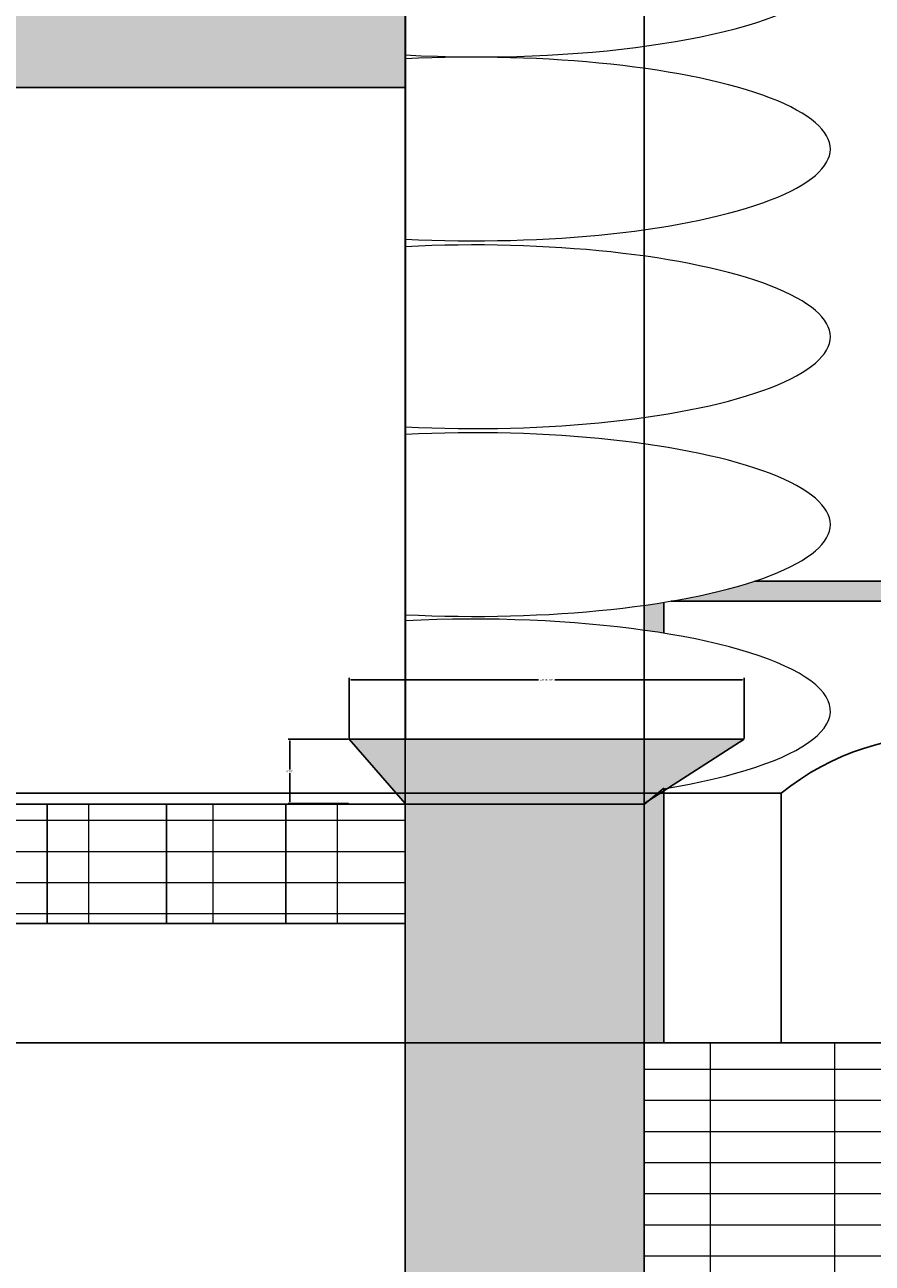
# Model space of a CAD drawing. Units: inches. Extents: x 484 to 1264, y 95 to 991.
# Tile 4 of 8: x 794 to 879, y 374 to 499. Entities that reach past the tile are written whole.
import ezdxf

# ---------------------------------------------------------------- set-up
doc = ezdxf.new("R2010")
doc.units = ezdxf.units.IN
doc.header["$MEASUREMENT"] = 0
for name, color, linetype, lineweight in [('A-ANNO-DIMS', 2, 'Continuous', 18), ('A-DOOR', 7, 'Continuous', 25), ('A-ELEV-TRIM', 7, 'Continuous', 18), ('A-WALL', 7, 'Continuous', 35), ('L-FENC', 7, 'Continuous', 25), ('L-FENC-GRIL-PATT', 6, 'Continuous', 13), ('L-GATE', 7, 'Continuous', 18)]:
    doc.layers.add(name, color=color, linetype=linetype, lineweight=lineweight)
doc.layers.add('A-ELEV-TRIM-PATT', color=40, linetype='Continuous', lineweight=13, true_color=0xe7c208)
doc.layers.add('L-FENC-PATT', color=34, linetype='Continuous', lineweight=13, true_color=0xa25420)
doc.styles.get("Standard").update_dxf_attribs({"font": 'arial.ttf'})
doc.dimstyles.get("Standard").update_dxf_attribs({"dimtxt": 0.18, "dimasz": 0.18, "dimexe": 0.18, "dimexo": 0.0625, "dimgap": 0.09, "dimtad": 0, "dimtih": 1, "dimtoh": 1, "dimdec": 4, "dimzin": 0, "dimdsep": 46, "dimtxsty": 'Standard', "dimcen": 0.09, "dimadec": 0, "dimazin": 0, "dimtfac": 1, "dimtdec": 4, "dimtofl": 0, "dimtmove": 0, "dimatfit": 3, "dimfxl": 1, "dimtolj": 1, "dimtzin": 0, "dimarcsym": 0})

# ---------------------------------------------------------------- blocks, each defined once
blk = doc.blocks.new('FENCE-PIER-CAP')
for p, q in [((5.628547385080537, 5.68e-14), (2.274e-13, 6.475381031596953)), ((2.274e-13, 6.475381031596953), (39.70506369136661, 6.475381031596953)), ((39.70506369136661, 6.475381031596953), (29.62854738508054, 0))]:
    blk.add_line(p, q)
blk = doc.blocks.new('*D14')
at = {"layer": 'A-ANNO-DIMS', "color": 0, "lineweight": -2, "transparency": 16777216}
for p, q in [((826.1861632675918, 426.9765617672598), (826.1861632675918, 433.0498213209647)), ((865.8912269589581, 426.9765617672598), (865.8912269589581, 433.0498213209647)), ((826.3661632675917, 432.8698213209647), (845.2181971596598, 432.8698213209647)), ((865.7112269589582, 432.8698213209647), (846.8591930668903, 432.8698213209647))]:
    blk.add_line(p, q, dxfattribs=at)
at = {"layer": 'A-ANNO-DIMS', "color": 0, "transparency": 16777216}
for points in [[(826.3661632675917, 432.8998213209647), (826.3661632675917, 432.8398213209648), (826.1861632675918, 432.8698213209647)], [(865.7112269589582, 432.8998213209647), (865.7112269589582, 432.8398213209648), (865.8912269589581, 432.8698213209647)]]:
    blk.add_solid(points, dxfattribs=at)
at = {"layer": 'Defpoints', "color": 0, "transparency": 16777216}
for p in [(865.8912269589581, 432.8698213209647), (826.1861632675918, 426.9140617672598), (865.8912269589581, 426.9140617672598)]:
    blk.add_point(p, dxfattribs=at)
at = {"layer": 'A-ANNO-DIMS', "color": 0, "transparency": 16777216, "insert": (846.038695113275, 432.8698213209647), "char_height": 0.18, "attachment_point": 5}
blk.add_mtext('\\A1;CAP 40 TYP.', dxfattribs=at)
blk = doc.blocks.new('*D15')
at = {"layer": 'A-ANNO-DIMS', "color": 0, "lineweight": -2, "transparency": 16777216}
for p, q in [((826.1236632675922, 426.9140617672601), (820.0504037138879, 426.9140617672601)), ((820.2304037138878, 426.73406176726), (820.2304037138878, 423.8582743892514)), ((820.2304037138878, 420.6186807356631), (820.2304037138878, 423.4944681136717)), ((826.1236632675922, 420.4386807356631), (820.0504037138879, 420.4386807356631))]:
    blk.add_line(p, q, dxfattribs=at)
at = {"layer": 'A-ANNO-DIMS', "color": 0, "transparency": 16777216}
for points in [[(820.2004037138877, 426.73406176726), (820.2604037138877, 426.73406176726), (820.2304037138878, 426.9140617672601)], [(820.2004037138877, 420.6186807356631), (820.2604037138877, 420.6186807356631), (820.2304037138878, 420.4386807356631)]]:
    blk.add_solid(points, dxfattribs=at)
at = {"layer": 'Defpoints', "color": 0, "transparency": 16777216}
for p in [(820.2304037138878, 426.9140617672601), (826.1861632675923, 426.9140617672601), (826.1861632675923, 420.4386807356631)]:
    blk.add_point(p, dxfattribs=at)
at = {"layer": 'A-ANNO-DIMS', "color": 0, "transparency": 16777216, "insert": (820.2304037138877, 423.6763712514612), "char_height": 0.18, "attachment_point": 5}
blk.add_mtext('\\A1;6 TYP.', dxfattribs=at)
blk = doc.blocks.new('*D16')
at = {"layer": 'A-ANNO-DIMS', "color": 0, "lineweight": -2, "transparency": 16777216}
for p, q in [((639.814711, 408.3220909999999), (639.814711, 94.79138999999998)), ((999.8147109999999, 318.322091), (999.8147109999999, 94.79138999999998)), ((639.9947109999999, 94.97139), (819.5262321459754, 94.97139)), ((999.634711, 94.97139), (820.1031898540245, 94.97139))]:
    blk.add_line(p, q, dxfattribs=at)
at = {"layer": 'A-ANNO-DIMS', "color": 0, "transparency": 16777216}
for points in [[(639.9947109999999, 95.00139), (639.9947109999999, 94.94139), (639.814711, 94.97139)], [(999.634711, 95.00139), (999.634711, 94.94139), (999.8147109999999, 94.97139)]]:
    blk.add_solid(points, dxfattribs=at)
at = {"layer": 'Defpoints', "color": 0, "transparency": 16777216}
for p in [(639.814711, 408.3845909999999), (999.8147109999999, 318.384591), (999.8147109999999, 94.97139)]:
    blk.add_point(p, dxfattribs=at)
at = {"layer": 'A-ANNO-DIMS', "color": 0, "transparency": 16777216, "insert": (819.814711, 94.97139), "char_height": 0.18, "attachment_point": 5}
blk.add_mtext('\\A1;360', dxfattribs=at)
blk = doc.blocks.new('*D18')
at = {"layer": 'A-ANNO-DIMS', "color": 0, "lineweight": -2, "transparency": 16777216}
for p, q in [((999.8772110000004, 501.3845910000002), (1264.083232000001, 501.3845910000003)), ((1263.903232000001, 501.2045910000002), (1263.903232000001, 404.0664941377902)), ((1263.903232000001, 306.5645910000002), (1263.903232000001, 403.7026878622103)), ((595.3846180000002, 306.3845910000001), (1264.083232000001, 306.3845910000002))]:
    blk.add_line(p, q, dxfattribs=at)
at = {"layer": 'A-ANNO-DIMS', "color": 0, "transparency": 16777216}
for points in [[(1263.873232000001, 501.2045910000002), (1263.933232000001, 501.2045910000002), (1263.903232000001, 501.3845910000003)], [(1263.873232000001, 306.5645910000002), (1263.933232000001, 306.5645910000002), (1263.903232000001, 306.3845910000002)]]:
    blk.add_solid(points, dxfattribs=at)
at = {"layer": 'Defpoints', "color": 0, "transparency": 16777216}
for p in [(999.8147110000004, 501.3845910000002), (1263.903232000001, 501.3845910000003), (595.3221180000002, 306.3845910000001)]:
    blk.add_point(p, dxfattribs=at)
at = {"layer": 'A-ANNO-DIMS', "color": 0, "transparency": 16777216, "insert": (1263.903232, 403.8845909999998), "char_height": 0.18, "attachment_point": 5}
blk.add_mtext('\\A1;195', dxfattribs=at)
blk = doc.blocks.new('*D29')
at = {"layer": 'A-ANNO-DIMS', "color": 0, "lineweight": -2, "transparency": 16777216}
for p, q in [((831.8147109999999, 906.322091), (831.8147109999999, 94.79139000000008)), ((784.302445, 819.993689), (784.302445, 94.79139000000008)), ((784.4824449999999, 94.97139), (807.6786257489769, 94.97139)), ((831.634711, 94.97139), (808.438530251023, 94.97139))]:
    blk.add_line(p, q, dxfattribs=at)
at = {"layer": 'A-ANNO-DIMS', "color": 0, "transparency": 16777216}
for points in [[(784.4824449999999, 95.00139), (784.4824449999999, 94.94139), (784.302445, 94.97139)], [(831.634711, 95.00139), (831.634711, 94.94139), (831.8147109999999, 94.97139)]]:
    blk.add_solid(points, dxfattribs=at)
at = {"layer": 'Defpoints', "color": 0, "transparency": 16777216}
for p in [(831.8147109999999, 906.3845909999999), (784.302445, 820.0561889999999), (831.8147109999999, 94.97139)]:
    blk.add_point(p, dxfattribs=at)
at = {"layer": 'A-ANNO-DIMS', "color": 0, "transparency": 16777216, "insert": (808.0585779999999, 94.97139), "char_height": 0.18, "attachment_point": 5}
blk.add_mtext('\\A1;47.51', dxfattribs=at)
blk = doc.blocks.new('*D46')
at = {"layer": 'A-ANNO-DIMS', "color": 0, "lineweight": -2, "transparency": 16777216}
for p, q in [((779.907407, 470.825236), (779.907407, 991.109014)), ((780.0874069999999, 990.929014), (805.4847288499319, 990.929014)), ((831.634711, 990.929014), (806.2373891500682, 990.929014)), ((831.8147109999999, 492.447091), (831.8147109999999, 991.109014))]:
    blk.add_line(p, q, dxfattribs=at)
at = {"layer": 'A-ANNO-DIMS', "color": 0, "transparency": 16777216}
for points in [[(780.0874069999999, 990.959014), (780.0874069999999, 990.899014), (779.907407, 990.929014)], [(831.634711, 990.959014), (831.634711, 990.899014), (831.8147109999999, 990.929014)]]:
    blk.add_solid(points, dxfattribs=at)
at = {"layer": 'Defpoints', "color": 0, "transparency": 16777216}
for p in [(831.8147109999999, 990.929014), (831.8147109999999, 492.3845909999999), (779.907407, 470.762736)]:
    blk.add_point(p, dxfattribs=at)
at = {"layer": 'A-ANNO-DIMS', "color": 0, "transparency": 16777216, "insert": (805.861059, 990.929014), "char_height": 0.18, "attachment_point": 5}
blk.add_mtext('\\A1;51.91', dxfattribs=at)
blk = doc.blocks.new('*D48')
at = {"layer": 'A-ANNO-DIMS', "color": 0, "lineweight": -2, "transparency": 16777216}
for p, q in [((831.7522110000004, 492.3845910000002), (484.1461180000004, 492.3845910000001)), ((484.3261180000005, 492.2045910000001), (484.3261180000005, 481.75556663779)), ((484.3261180000005, 470.9427360000002), (484.3261180000005, 481.3917603622102)), ((779.8449070000004, 470.7627360000002), (484.1461180000004, 470.7627360000001))]:
    blk.add_line(p, q, dxfattribs=at)
at = {"layer": 'A-ANNO-DIMS', "color": 0, "transparency": 16777216}
for points in [[(484.2961180000004, 492.2045910000001), (484.3561180000004, 492.2045910000001), (484.3261180000005, 492.3845910000001)], [(484.2961180000004, 470.9427360000002), (484.3561180000004, 470.9427360000002), (484.3261180000005, 470.7627360000001)]]:
    blk.add_solid(points, dxfattribs=at)
at = {"layer": 'Defpoints', "color": 0, "transparency": 16777216}
for p in [(484.3261180000005, 492.3845910000001), (831.8147110000004, 492.3845910000002), (779.9074070000004, 470.7627360000002)]:
    blk.add_point(p, dxfattribs=at)
at = {"layer": 'A-ANNO-DIMS', "color": 0, "transparency": 16777216, "insert": (484.3261180000005, 481.5736634999999), "char_height": 0.18, "attachment_point": 5}
blk.add_mtext('\\A1;21.62', dxfattribs=at)
blk = doc.blocks.new('*D51')
at = {"layer": 'A-ANNO-DIMS', "color": 0, "lineweight": -2, "transparency": 16777216}
for p, q in [((869.5523070000005, 421.4725140000002), (484.1461180000004, 421.4725140000001)), ((484.3261180000004, 421.2925140000001), (484.3261180000005, 370.1105170293316)), ((484.3261180000005, 318.5645910000001), (484.3261180000005, 369.7465879706685)), ((855.7522110000004, 318.3845910000001), (484.1461180000004, 318.384591))]:
    blk.add_line(p, q, dxfattribs=at)
at = {"layer": 'A-ANNO-DIMS', "color": 0, "transparency": 16777216}
for points in [[(484.2961180000004, 421.2925140000001), (484.3561180000003, 421.2925140000001), (484.3261180000004, 421.4725140000001)], [(484.2961180000004, 318.5645910000001), (484.3561180000004, 318.5645910000001), (484.3261180000005, 318.384591)]]:
    blk.add_solid(points, dxfattribs=at)
at = {"layer": 'Defpoints', "color": 0, "transparency": 16777216}
for p in [(484.3261180000004, 421.4725140000001), (869.6148070000004, 421.4725140000002), (855.8147110000004, 318.3845910000001)]:
    blk.add_point(p, dxfattribs=at)
at = {"layer": 'A-ANNO-DIMS', "color": 0, "transparency": 16777216, "insert": (484.3261180000004, 369.9285524999999), "char_height": 0.18, "attachment_point": 5}
blk.add_mtext('\\A1;103.09', dxfattribs=at)
blk = doc.blocks.new('*D54')
at = {"layer": 'A-ANNO-DIMS', "color": 0, "lineweight": -2, "transparency": 16777216}
for p, q in [((831.8147109999999, 420.501181), (831.8147109999999, 991.109014)), ((831.9947109999999, 990.929014), (843.5946223233287, 990.929014)), ((855.634711, 990.929014), (844.0347996766712, 990.929014)), ((855.814711, 420.501181), (855.814711, 991.109014))]:
    blk.add_line(p, q, dxfattribs=at)
at = {"layer": 'A-ANNO-DIMS', "color": 0, "transparency": 16777216}
for points in [[(831.9947109999999, 990.959014), (831.9947109999999, 990.899014), (831.8147109999999, 990.929014)], [(855.634711, 990.959014), (855.634711, 990.899014), (855.814711, 990.929014)]]:
    blk.add_solid(points, dxfattribs=at)
at = {"layer": 'Defpoints', "color": 0, "transparency": 16777216}
for p in [(855.814711, 990.929014), (831.8147109999999, 420.4386809999999), (855.814711, 420.4386809999999)]:
    blk.add_point(p, dxfattribs=at)
at = {"layer": 'A-ANNO-DIMS', "color": 0, "transparency": 16777216, "insert": (843.8147109999999, 990.929014), "char_height": 0.18, "attachment_point": 5}
blk.add_mtext('\\A1;24', dxfattribs=at)
blk = doc.blocks.new('*D57')
at = {"layer": 'A-ANNO-DIMS', "color": 0, "lineweight": -2, "transparency": 16777216}
for p, q in [((855.814711, 396.447091), (855.814711, 991.109014)), ((855.9947109999999, 990.929014), (879.5919824870394, 990.929014)), ((903.6347110000002, 990.929014), (880.0374395129605, 990.929014)), ((903.814711, 396.447091), (903.814711, 991.109014))]:
    blk.add_line(p, q, dxfattribs=at)
at = {"layer": 'A-ANNO-DIMS', "color": 0, "transparency": 16777216}
for points in [[(855.9947109999999, 990.959014), (855.9947109999999, 990.899014), (855.814711, 990.929014)], [(903.6347110000002, 990.959014), (903.6347110000002, 990.899014), (903.814711, 990.929014)]]:
    blk.add_solid(points, dxfattribs=at)
at = {"layer": 'Defpoints', "color": 0, "transparency": 16777216}
for p in [(903.814711, 990.929014), (855.814711, 396.384591), (903.814711, 396.384591)]:
    blk.add_point(p, dxfattribs=at)
at = {"layer": 'A-ANNO-DIMS', "color": 0, "transparency": 16777216, "insert": (879.814711, 990.929014), "char_height": 0.18, "attachment_point": 5}
blk.add_mtext('\\A1;48', dxfattribs=at)
blk = doc.blocks.new('*D58')
at = {"layer": 'A-ANNO-DIMS', "color": 0, "lineweight": -2, "transparency": 16777216}
for p, q in [((855.7522110000004, 396.3845910000003), (484.1461180000004, 396.3845910000001)), ((484.3261180000004, 396.2045910000002), (484.3261180000005, 363.56649413779)), ((484.3261180000005, 330.5645910000001), (484.3261180000005, 363.2026878622101)), ((855.7522110000004, 330.3845910000001), (484.1461180000004, 330.3845910000001))]:
    blk.add_line(p, q, dxfattribs=at)
at = {"layer": 'A-ANNO-DIMS', "color": 0, "transparency": 16777216}
for points in [[(484.2961180000004, 396.2045910000002), (484.3561180000003, 396.2045910000002), (484.3261180000004, 396.3845910000001)], [(484.2961180000004, 330.5645910000001), (484.3561180000004, 330.5645910000001), (484.3261180000005, 330.3845910000001)]]:
    blk.add_solid(points, dxfattribs=at)
at = {"layer": 'Defpoints', "color": 0, "transparency": 16777216}
for p in [(484.3261180000004, 396.3845910000001), (855.8147110000004, 396.3845910000003), (855.8147110000004, 330.3845910000001)]:
    blk.add_point(p, dxfattribs=at)
at = {"layer": 'A-ANNO-DIMS', "color": 0, "transparency": 16777216, "insert": (484.3261180000004, 363.3845909999998), "char_height": 0.18, "attachment_point": 5}
blk.add_mtext('\\A1;66', dxfattribs=at)
blk = doc.blocks.new('*D61')
at = {"layer": 'A-ANNO-DIMS', "color": 0, "lineweight": -2, "transparency": 16777216}
for p, q in [((855.814711, 396.447091), (855.814711, 991.109014)), ((855.9947109999999, 990.929014), (881.2626698690314, 990.929014)), ((907.3184050000001, 990.929014), (882.0504461309687, 990.929014)), ((907.498405, 442.840754), (907.498405, 991.1090139999998))]:
    blk.add_line(p, q, dxfattribs=at)
at = {"layer": 'A-ANNO-DIMS', "color": 0, "transparency": 16777216}
for points in [[(855.9947109999999, 990.959014), (855.9947109999999, 990.899014), (855.814711, 990.929014)], [(907.3184050000001, 990.959014), (907.3184050000001, 990.899014), (907.498405, 990.929014)]]:
    blk.add_solid(points, dxfattribs=at)
at = {"layer": 'Defpoints', "color": 0, "transparency": 16777216}
for p in [(907.498405, 990.929014), (907.498405, 442.7782539999999), (855.814711, 396.384591)]:
    blk.add_point(p, dxfattribs=at)
at = {"layer": 'A-ANNO-DIMS', "color": 0, "transparency": 16777216, "insert": (881.656558, 990.929014), "char_height": 0.18, "attachment_point": 5}
blk.add_mtext('\\A1;51.68', dxfattribs=at)

msp = doc.modelspace()

# ---------------------------------------------------------------- hatches: boundary and pattern name
at = {"layer": 'A-ELEV-TRIM-PATT'}
h = msp.add_hatch(color=256, dxfattribs=at)
h.dxf.hatch_style = 1
h.paths.add_polyline_path([(791.3604632189817, 737.6508125955456), (707.0379608801577, 737.6508125955456), (707.0379608801577, 581.2764007961791), (791.3604632189817, 581.2764007961791)])
h.paths.add_polyline_path([(789.3604632189817, 735.6508125955456), (789.3604632189817, 583.2764007961791), (709.0379608801576, 583.2764007961791), (709.0379608801576, 735.6508125955456)], flags=16)
h.paths.add_polyline_path([(850.1751791371953, 699.3334200613348), (840.6400557475826, 699.3334200613348), (840.6400557475826, 681.6081848608055), (850.1751791371953, 681.6081848608055)])
h.paths.add_polyline_path([(850.9809155201601, 648.8446729214583), (839.9452998180949, 648.8446729214583), (839.9452998180949, 628.2142842352996), (850.9809155201601, 628.2142842352996)])
h.paths.add_polyline_path([(849.2080120719693, 595.8058680326312), (838.5283820280656, 595.8058680326312), (838.5283820280656, 577.665356669208), (849.2080120719693, 577.665356669208)])
h.paths.add_polyline_path([(723.4575003799, 950.0790139985864), (709.0682911431468, 950.0790139985864), (709.0682911431468, 889.1187126845098), (723.4575003799, 889.1187126845098)])
h.paths.add_polyline_path([(750.5092145489798, 950.0790139985864), (736.1200053122265, 950.0790139985864), (736.1200053122265, 889.1187126845098), (750.5092145489798, 889.1187126845098)])
h.paths.add_polyline_path([(775.2586596621131, 950.0790139985864), (760.8694504253598, 950.0790139985864), (760.8694504253598, 889.1187126845098), (775.2586596621131, 889.1187126845098)])
h.paths.add_polyline_path([(759.8947585294499, 859.8728276012089), (737.9776673698088, 859.8728276012089), (737.9776673698088, 820.0561886043143), (759.8947585294499, 820.0561886043143)])
h.paths.add_polyline_path([(757.89475852945, 822.0561886043142), (739.9776673698088, 822.0561886043142), (739.9776673698088, 857.8728276012089), (757.89475852945, 857.8728276012089)], flags=16)
h.paths.add_polyline_path([(806.2195360287933, 859.8728276012089), (784.302444869152, 859.8728276012089), (784.302444869152, 820.0561886043143), (806.2195360287933, 820.0561886043143)])
h.paths.add_polyline_path([(786.302444869152, 857.8728276012089), (804.2195360287932, 857.8728276012089), (804.2195360287932, 822.0561886043142), (786.302444869152, 822.0561886043142)], flags=16)
h.paths.add_polyline_path([(711.5775266940199, 859.8728276012089), (689.6604355343788, 859.8728276012089), (689.6604355343788, 820.0561886043143), (711.5775266940199, 820.0561886043143)])
h.paths.add_polyline_path([(709.57752669402, 822.0561886043142), (691.6604355343788, 822.0561886043142), (691.6604355343788, 857.8728276012089), (709.57752669402, 857.8728276012089)], flags=16)
h.paths.add_polyline_path([(831.8147106526719, 810.3845910111976), (663.814710652672, 810.3845910111976), (663.814710652672, 801.3845910111976), (831.8147106526719, 801.3845910111978)])
h.paths.add_polyline_path([(831.8147106526719, 501.3845910111976), (663.814710652672, 501.3845910111978), (663.814710652672, 492.3845910111977), (831.8147106526719, 492.3845910111977)])
h.paths.add_polyline_path([(779.9074070481965, 470.7627364727195), (732.7744315549462, 470.7627364727195), (732.7744315549462, 420.3845910111978), (734.7744315549462, 420.3845910111978), (734.7744315549462, 468.7627364727195), (777.9074070481965, 468.7627364727195), (777.9074070481965, 420.3845910111978), (779.9074070481965, 420.3845910111978)])
h.paths.add_polyline_path([(779.9074070481965, 420.3845910111978), (777.9074070481965, 420.3845910111978), (777.9074070481965, 414.1588149678183), (771.814710652672, 414.1588149678181), (771.814710652672, 412.1588149678181), (779.9074070481965, 412.1588149678181)])
h = msp.add_hatch(color=256, dxfattribs=at)
h.dxf.hatch_style = 1
h.paths.add_polyline_path([(629.3986341127111, 426.8599720427947), (589.6935704213448, 426.8599720427947), (595.3221178064251, 420.3845910111978), (619.3221178064251, 420.3845910111978)])
edge = h.paths.add_edge_path()
edge.add_line((857.8147106526719, 421.9731071829778), (857.8147106526719, 421.9373150679256))
edge.add_ellipse((838.7194759063842, 429.7417652989397), major_axis=(-35.82412926401594, 0), ratio=0.257481448966652, start_angle=157.769579789742, end_angle=158.4161923974365)
edge.add_line((858.2613839007333, 422.0109643562563), (865.8912269589578, 426.9140617672601))
edge.add_line((865.8912269589578, 426.9140617672601), (826.1861632675914, 426.9140617672601))
edge.add_line((826.1861632675914, 426.9140617672601), (831.8617266623419, 420.3845910111978))
edge.add_line((831.8617266623419, 420.3845910111978), (855.7305401632568, 420.3845910111978))
edge.add_line((855.7305401632568, 420.3845910111978), (856.344544620657, 420.7791631724401))
edge.add_line((856.344544620657, 420.7791631724401), (857.8147106526719, 421.9731071829778))
h.paths.add_polyline_path([(1009.891226958958, 426.8599720427946), (970.1861632675917, 426.8599720427946), (975.814710652672, 420.3845910111978), (999.8147106526721, 420.3845910111977)])
h.paths.add_polyline_path([(857.8147106526719, 421.7239227448598), (856.3445446206568, 420.7791631724401), (855.8147106526719, 420.3488770150404), (855.8147106526719, 396.3845910111981), (857.8147106526719, 396.3845910111981)])
edge = h.paths.add_edge_path()
edge.add_ellipse((838.7194759063842, 448.4615448867479), major_axis=(-35.82412926401594, 0), ratio=0.257481448966652, start_angle=154.6310860812245, end_angle=157.7695797897421, ccw=False)
edge.add_line((855.8147106526719, 440.3554940259931), (855.8147106526719, 437.8478161596945))
edge.add_ellipse((838.7194759063842, 429.7417652989397), major_axis=(-35.82412926401594, 0), ratio=0.257481448966652, start_angle=202.230420210258, end_angle=205.3689139187756, ccw=False)
edge.add_line((857.8147106526719, 437.5462155299538), (857.8147106526719, 440.6570946557339))
edge = h.paths.add_edge_path()
edge.add_line((907.4984049521273, 442.7782537442242), (866.935916483663, 442.7782537442242))
edge.add_ellipse((838.7194759063842, 448.4615448867479), major_axis=(-35.82412926401594, 0), ratio=0.257481448966652, start_angle=158.8134614821794, end_angle=168.6119836679537, ccw=False)
edge.add_line((858.5419953103798, 440.7782537442242), (905.4984049521271, 440.7782537442242))
edge.add_line((905.4984049521271, 440.7782537442242), (905.4984049521271, 418.756158794456))
edge.add_line((905.4984049521271, 418.756158794456), (907.4984049521273, 416.8218026381525))
edge.add_line((907.4984049521273, 416.8218026381525), (907.4984049521273, 442.7782537442242))
at = {"layer": 'L-FENC-GRIL-PATT'}
h = msp.add_hatch(dxfattribs=at)
h.set_pattern_fill('GRATE', color=256, scale=100)
h.set_pattern_definition([(0, (0, 0), (0, 3.125), []), (90, (0, 0), (-12.5, 8e-16), [])])
h.paths.add_polyline_path([(974.8147106526721, 396.3845910111977), (927.8147106526721, 396.3845910111978), (927.814710652672, 330.3845910111977), (974.8147106526719, 330.3845910111978)])
h.paths.add_polyline_path([(903.8147106526721, 396.3845910111981), (855.8147106526719, 396.3845910111981), (855.8147106526719, 330.3845910111977), (903.814710652672, 330.3845910111976)])
h.paths.add_polyline_path([(819.814710652672, 420.3845910111978), (807.8147106526721, 420.3845910111978), (807.8147106526721, 408.3845910111977), (819.8147106526718, 408.3845910111977)])
h.paths.add_polyline_path([(807.8147106526721, 420.3845910111978), (795.814710652672, 420.3845910111978), (795.8147106526719, 408.3845910111978), (807.8147106526721, 408.3845910111977)])
h.paths.add_polyline_path([(795.814710652672, 420.3845910111978), (783.814710652672, 420.3845910111978), (783.8147106526719, 408.3845910111978), (795.8147106526719, 408.3845910111978)])
h.paths.add_polyline_path([(831.8147106526719, 420.3845910111978), (819.814710652672, 420.3845910111978), (819.8147106526718, 408.3845910111977), (831.8147106526719, 408.3845910111977)])
h.paths.add_polyline_path([(783.814710652672, 420.3845910111978), (779.9104622014929, 420.3845910111978), (779.9104622014929, 412.1379508589634), (771.814710652672, 412.1379508589634), (771.814710652672, 408.3845910111978), (783.8147106526719, 408.3845910111978)])
h.paths.add_polyline_path([(777.9104622014929, 420.3845910111978), (771.814710652672, 420.3845910111978), (771.814710652672, 414.1379508589634), (777.9104622014929, 414.1379508589634)], flags=17)
h.paths.add_polyline_path([(723.8147106526721, 420.3845910111978), (711.8147106526721, 420.3845910111978), (711.814710652672, 408.3845910111978), (723.8147106526721, 408.3845910111978)])
h.paths.add_polyline_path([(711.8147106526721, 420.3845910111978), (699.814710652672, 420.3845910111978), (699.814710652672, 408.3845910111978), (711.814710652672, 408.3845910111978)])
h.paths.add_polyline_path([(699.814710652672, 420.3845910111978), (687.814710652672, 420.3845910111978), (687.814710652672, 408.3845910111978), (699.814710652672, 408.3845910111978)])
h.paths.add_polyline_path([(687.814710652672, 420.3845910111978), (675.814710652672, 420.3845910111978), (675.814710652672, 408.3845910111978), (687.814710652672, 408.3845910111978)])
h.paths.add_polyline_path([(675.814710652672, 420.3845910111978), (663.8147106526719, 420.3845910111978), (663.814710652672, 408.3845910111977), (675.814710652672, 408.3845910111978)])
h.paths.add_polyline_path([(639.814710652672, 420.3845910111978), (631.3221178064251, 420.3845910111978), (631.3221178064249, 408.3845910111977), (639.814710652672, 408.3845910111977)])
h.paths.add_polyline_path([(631.3221178064251, 420.3845910111978), (619.3221178064249, 420.3845910111978), (619.3221178064249, 408.3845910111977), (631.3221178064249, 408.3845910111977)])
at = {"layer": 'L-FENC-PATT'}
h = msp.add_hatch(color=256, dxfattribs=at)
h.dxf.hatch_style = 1
h.paths.add_polyline_path([(619.3221178064251, 420.3845910111978), (595.3221178064251, 420.3845910111978), (595.3221178064248, 306.3845910111977), (855.8147106526719, 306.3845910111977), (855.8147106526719, 420.3845910111978), (831.8147106526719, 420.3845910111978), (831.8147106526719, 330.3845910111977), (771.8147106526721, 330.3845910111976), (771.814710652672, 420.3845910111978), (723.8147106526721, 420.3845910111978), (723.814710652672, 330.3845910111976), (619.3221178064249, 330.3845910111977)])
h.paths.add_polyline_path([(999.8147106526721, 420.3845910111977), (975.814710652672, 420.3845910111978), (975.8147106526719, 318.3845910111977), (999.8147106526719, 318.3845910111977)])

# ---------------------------------------------------------------- linework, layer by layer
at = {"layer": 'A-DOOR'}
msp.add_line((869.6148065231833, 421.472513971546), (869.6148065231833, 396.3845910111981), dxfattribs=at)
for points in [[(907.4984049521273, 416.8218026381524), (907.4984049521273, 442.7782537442242), (866.935916483663, 442.7782537442242)], [(857.8147106526719, 440.6570946557339), (857.8147106526719, 437.5462155299538)], [(905.4984049521271, 418.7561587944559), (905.4984049521271, 440.7782537442242), (858.5419953103798, 440.7782537442242)], [(855.8147106526719, 440.3554940259931), (855.8147106526719, 437.8478161596945)], [(857.8147106526719, 421.9731071829778), (857.8147106526719, 396.3845910111981)], [(855.8147106526719, 420.3845910111978), (855.8147106526719, 396.3845910111981), (903.8147106526721, 396.3845910111981)]]:
    msp.add_lwpolyline(points, dxfattribs=at)
msp.add_arc((886.0837479452722, 401.0921263196208), 26.20279054617937, 47.41507843545075, 128.9409124410971, dxfattribs=at)
at = {"layer": 'A-ELEV-TRIM'}
msp.add_line((831.8147106526719, 492.3845910111977), (663.814710652672, 492.3845910111977), dxfattribs=at)
for centre, start_param, end_param in [((839.159623118232, 504.6688599429044), 1.364305070234511, 2.777549809473754), ((838.7194759063842, 486.189488100109), 1.376841942592971, 4.906343364586614), ((838.7194759063842, 467.3283807948546), 1.376841942592971, 4.906343364586614), ((838.7194759063842, 448.4615448867479), 1.376841942592971, 4.906343364586614), ((838.7194759063842, 429.7417652989397), 2.131155702969735, 4.906343364586614)]:
    msp.add_ellipse(centre, major_axis=(-35.82412926401594, 0), ratio=0.257481448966652, start_param=start_param, end_param=end_param, dxfattribs=at)
at = {"layer": 'A-WALL'}
for p, q in [((831.8147106526719, 906.3845910111979), (831.8147106526719, 491.1648903637863)), ((831.8147106526719, 491.1648903637863), (831.8147106526717, 426.9140617672601))]:
    msp.add_line(p, q, dxfattribs=at)
at = {"layer": 'L-FENC'}
for p, q in [((855.8586871738107, 420.3845910111977), (857.8147106526719, 421.9731071829778)), ((855.8147106526719, 420.3845910111978), (663.814710652672, 420.3845910111978)), ((795.814710652672, 420.3845910111978), (795.8147106526719, 408.3845910111978)), ((807.8147106526721, 420.3845910111978), (807.8147106526721, 408.3845910111978)), ((819.814710652672, 420.3845910111978), (819.8147106526718, 408.3845910111978)), ((831.8586871738107, 420.3845910111978), (831.8147106526717, 420.4386807356631)), ((831.8147106526719, 420.4386807356631), (831.8147106526719, 330.3845910111976)), ((855.8147106526719, 420.3845910111978), (855.8147106526719, 306.3845910111977)), ((831.8147106526719, 408.3845910111977), (771.8147106526721, 408.3845910111978))]:
    msp.add_line(p, q, dxfattribs=at)
at = {"layer": 'L-GATE'}
msp.add_line((903.8147106526721, 396.3845910111979), (855.8147106526719, 396.3845910111981), dxfattribs=at)

# ---------------------------------------------------------------- block references
at = {"layer": 'L-FENC'}
msp.add_blockref('FENCE-PIER-CAP', (826.1861632675916, 420.4386807356629), dxfattribs=at)

# ---------------------------------------------------------------- dimensions: what is measured, and where the dimension line sits
at = {"layer": 'A-ANNO-DIMS'}
for base, p1, p2, override, picture, middle in [((831.8147109999999, 990.929014), (779.907407, 470.762736), (831.8147109999999, 492.3845909999999), {"dimdec": 2, "dimlfac": 1, "dimrnd": 0, "dimzin": 0, "dimdsep": 46, "dimlunit": 2}, '*D46', (805.861059, 990.929014)), ((855.814711, 990.929014), (831.8147109999999, 420.4386809999999), (855.814711, 420.4386809999999), {"dimdec": 0, "dimlfac": 1, "dimrnd": 0, "dimzin": 0, "dimdsep": 46, "dimlunit": 2}, '*D54', (843.8147109999999, 990.929014)), ((903.814711, 990.929014), (855.814711, 396.384591), (903.814711, 396.384591), {"dimdec": 0, "dimlfac": 1, "dimrnd": 0, "dimzin": 0, "dimdsep": 46, "dimlunit": 2}, '*D57', (879.814711, 990.929014)), ((907.498405, 990.929014), (855.814711, 396.384591), (907.498405, 442.7782539999999), {"dimdec": 2, "dimlfac": 1, "dimrnd": 0, "dimzin": 0, "dimdsep": 46, "dimlunit": 2}, '*D61', (881.656558, 990.929014)), ((831.8147109999999, 94.97139), (784.302445, 820.0561889999999), (831.8147109999999, 906.3845909999999), {"dimdec": 2, "dimlfac": 1, "dimrnd": 0, "dimzin": 0, "dimdsep": 46, "dimlunit": 2}, '*D29', (808.0585779999999, 94.97139)), ((999.8147109999999, 94.97139), (639.814711, 408.3845909999999), (999.8147109999999, 318.384591), {"dimdec": 0, "dimlfac": 1, "dimrnd": 0, "dimzin": 0, "dimdsep": 46, "dimlunit": 2}, '*D16', (819.814711, 94.97139))]:
    dim = msp.add_linear_dim(base=base, p1=p1, p2=p2, dimstyle='Standard', override=override, dxfattribs=at)
    dim.commit()
    dim.dimension.update_dxf_attribs({"geometry": picture, "text_midpoint": middle})
for base, p1, p2, override, picture, middle in [((1263.903232000001, 501.3845910000003), (595.322118, 306.384591), (999.8147109999999, 501.3845909999999), {"dimdec": 0, "dimlfac": 1, "dimrnd": 0, "dimzin": 0, "dimdsep": 46, "dimlunit": 2}, '*D18', (1263.903232, 403.8845909999998)), ((484.3261180000005, 492.3845910000001), (779.907407, 470.762736), (831.8147109999999, 492.3845909999999), {"dimdec": 2, "dimlfac": 1, "dimrnd": 0, "dimzin": 0, "dimdsep": 46, "dimlunit": 2}, '*D48', (484.3261180000005, 481.5736634999999)), ((484.3261180000004, 421.4725140000001), (855.814711, 318.384591), (869.6148070000002, 421.4725139999999), {"dimdec": 2, "dimlfac": 1, "dimrnd": 0, "dimzin": 0, "dimdsep": 46, "dimlunit": 2}, '*D51', (484.3261180000004, 369.9285524999999)), ((484.3261180000004, 396.3845910000001), (855.814711, 330.384591), (855.814711, 396.384591), {"dimdec": 0, "dimlfac": 1, "dimrnd": 0, "dimzin": 0, "dimdsep": 46, "dimlunit": 2}, '*D58', (484.3261180000004, 363.3845909999998))]:
    dim = msp.add_linear_dim(base=base, p1=p1, p2=p2, angle=90, dimstyle='Standard', override=override, dxfattribs=at)
    dim.commit()
    dim.dimension.update_dxf_attribs({"geometry": picture, "text_midpoint": middle})
dim = msp.add_linear_dim(base=(865.8912269589581, 432.8698213209647), p1=(826.1861632675918, 426.9140617672598), p2=(865.8912269589581, 426.9140617672598), text='CAP <> TYP.', dimstyle='Standard', override={"dimdec": 0, "dimlfac": 1, "dimrnd": 0, "dimzin": 0, "dimdsep": 46, "dimlunit": 2}, dxfattribs=at)
dim.commit()
dim.dimension.update_dxf_attribs({"geometry": '*D14', "text_midpoint": (846.038695113275, 432.8698213209647)})
dim = msp.add_linear_dim(base=(820.2304037138878, 426.9140617672601), p1=(826.1861632675918, 420.4386807356629), p2=(826.1861632675918, 426.9140617672598), angle=90, text='<> TYP.', dimstyle='Standard', override={"dimdec": 0, "dimlfac": 1, "dimrnd": 0, "dimzin": 0, "dimdsep": 46, "dimlunit": 2}, dxfattribs=at)
dim.commit()
dim.dimension.update_dxf_attribs({"geometry": '*D15', "text_midpoint": (820.2304037138877, 423.6763712514612)})

doc.saveas('drawing.dxf')
